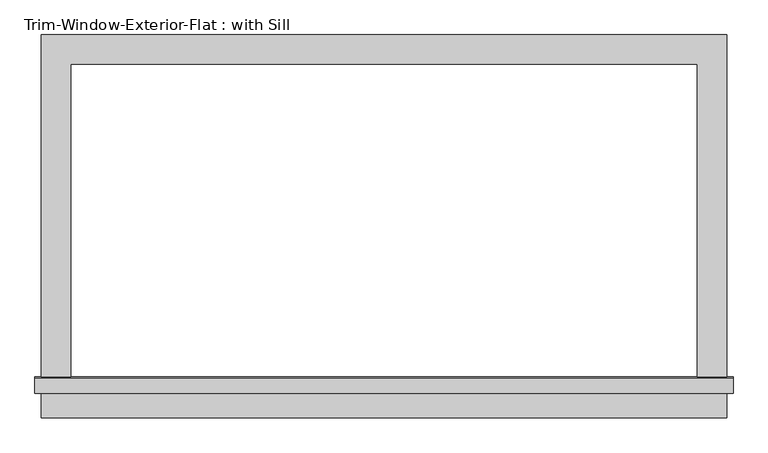
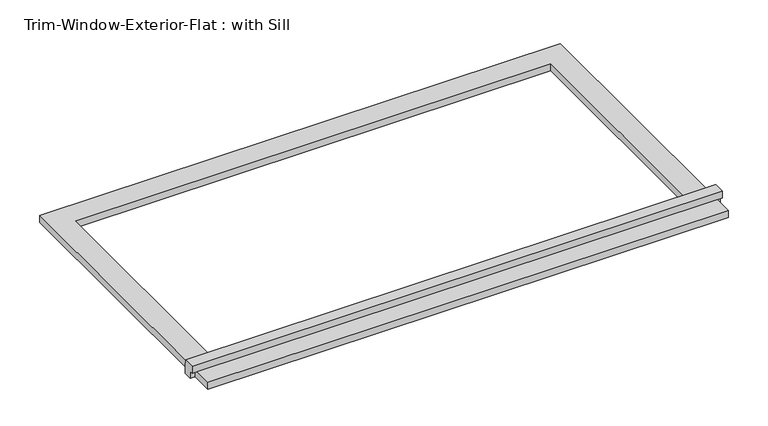
"""IFC4 building model written with IfcOpenShell, lengths in millimetres: proxy geometry, Trim-Window-Exterior-Flat : with Sill."""

from ifc_helpers import new_model, si_unit, frame, origin, origin_with_axes, place, context, project, spatial, polyline, outline, extrude, source, transform, mapped, element, save


def trim_window_exterior_flat_with_sill_a633738d(model_context):
    return source(origin(), model_context, "Body", "SweptSolid", [
        extrude(outline(polyline([(666.75, -631.7823709), (666.75, -688.9323709), (-666.75, -688.9323709), (-666.75, -631.7823709), (666.75, -631.7823709)])), origin_with_axes(), (0.0, 0.0, 1.0), 19.05),
        extrude(outline(polyline([(-641.35, 38.1), (-612.0580645, 38.1), (-609.6, 19.05), (-609.6, 0.0), (-631.7823709, 0.0), (-631.7823709, 19.05), (-641.35, 19.05), (-641.35, 38.1)])), frame((-679.45, 0.0, 0.0), z_axis=(1.0, 0.0, 0.0), x_axis=(0.0, 1.0, 0.0)), (0.0, 0.0, 1.0), 1358.9),
        extrude(outline(polyline([(-666.75, 57.15), (666.75, 57.15), (666.75, -609.6), (609.6, -609.6), (609.6, 0.0), (-609.6, 0.0), (-609.6, -609.6), (-666.75, -609.6), (-666.75, 57.15)])), origin_with_axes(), (0.0, 0.0, 1.0), 19.05),
    ])


if __name__ == "__main__":
    model = new_model("IFC4")
    model_context = context("Model", 3, world=origin())
    ifc_project = project(units=[si_unit("LENGTHUNIT", "METRE", prefix="MILLI")], contexts=[model_context])
    site = spatial("IfcSite", under=ifc_project)
    building = spatial("IfcBuilding", under=site)
    placement = place(None, origin())
    trim_window_exterior_flat_with_sill_shape = trim_window_exterior_flat_with_sill_a633738d(model_context)
    element("IfcBuildingElementProxy", 1, Name="Trim-Window-Exterior-Flat : with Sill", ObjectType="Trim-Window-Exterior-Flat : with Sill", at=placement, inside=building, context=model_context, shape_type="MappedRepresentation", body=[
        mapped(trim_window_exterior_flat_with_sill_shape, transform((0.0, 0.0, 0.0), x_axis=(1.0, 0.0, 0.0), y_axis=(0.0, 1.0, 0.0), z_axis=(0.0, 0.0, 1.0))),
    ])
    save(model, "model.ifc")

# Revit data of these elements
# Type "Trim-Window-Exterior-Flat : with Sill"
#   Trim Width = 0' - 2 1/4"
#   Trim Thickness_Picture Frame = 0' - 1 1/4"
#   Trim Thickness_with Sill = 0' - 0 3/4"
#   Sill Thickness = 0' - 1 1/4"
#   Opening Width [instance default] = 2' - 0"
#   Opening Height [instance default] = 3' - 0"
#   Default Elevation = 4' - 0"
#   Sill = yes
#   Picture Frame = no
#   Trim Material [instance default] = none
# Element 1 (IfcBuildingElementProxy, "Trim-Window-Exterior-Flat : with Sill")
#   Opening Width = 4' - 0"
#   Opening Height = 2' - 0"
#   Trim Material = Clad - White
#   Materials on its faces: "Clad - White"
# Materials
#   "Clad - White": class "Wood", colour RGB 242 242 238, transparency 0, Cost = 0
